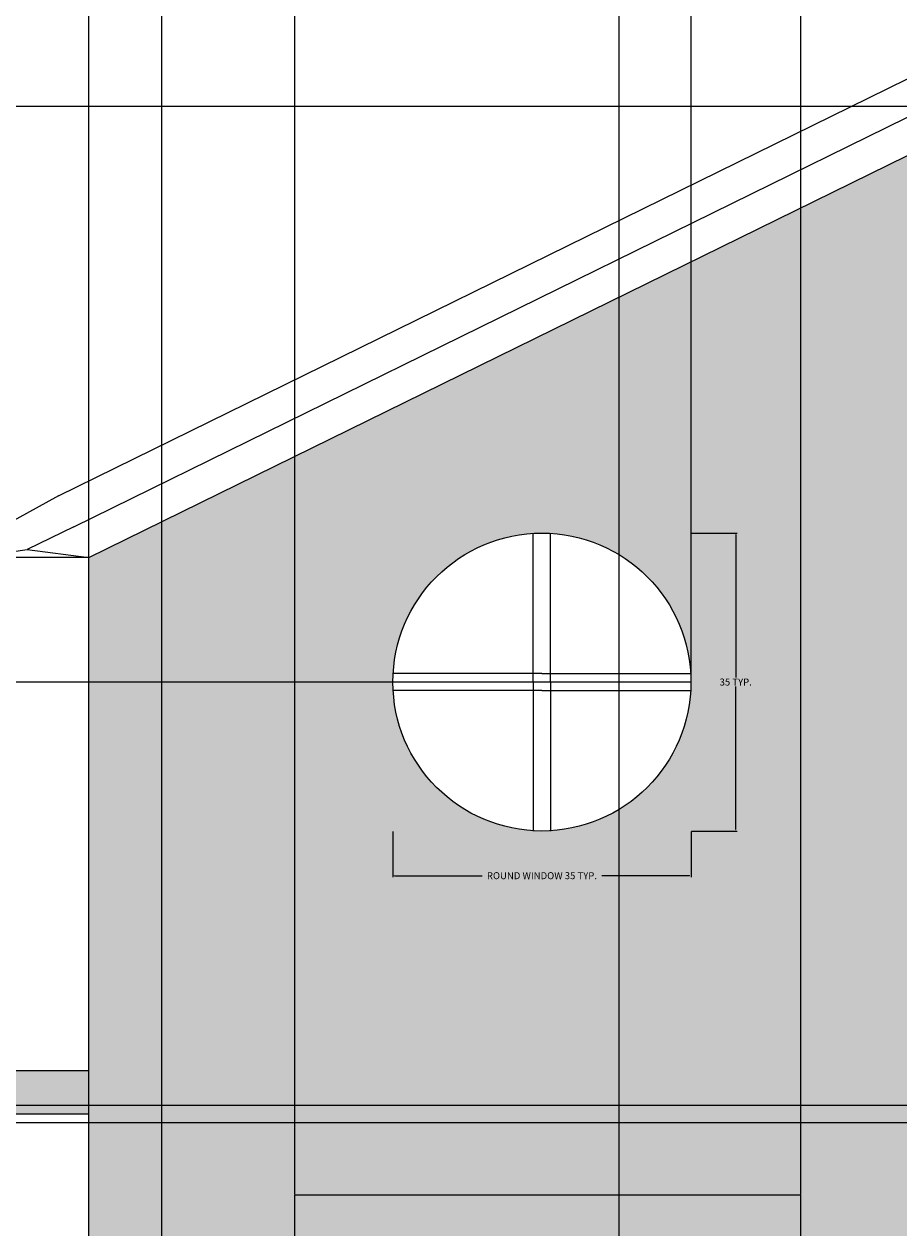
# Model space of a CAD drawing. Units: inches. Extents: x 36 to 594, y 79 to 831.
# Tile 21 of 30: x 87 to 189, y 590 to 730. Entities that reach past the tile are written whole.
import ezdxf

# ---------------------------------------------------------------- set-up
doc = ezdxf.new("R2010")
doc.units = ezdxf.units.IN
doc.header["$MEASUREMENT"] = 0
for name, color, linetype, lineweight in [('A-ANNO-DIMS', 2, 'Continuous', 18), ('A-ELEV', 7, 'Continuous', 25), ('A-ELEV-PATT', 8, 'Continuous', 13), ('A-GLAZ', 4, 'Continuous', 18)]:
    doc.layers.add(name, color=color, linetype=linetype, lineweight=lineweight)
doc.styles.get("Standard").update_dxf_attribs({"font": 'arial.ttf'})
doc.dimstyles.get("Standard").update_dxf_attribs({"dimtxt": 0.8125, "dimasz": 0.18, "dimexe": 0.18, "dimexo": 0.0625, "dimgap": 0.09, "dimtad": 0, "dimtih": 1, "dimtoh": 1, "dimdec": 4, "dimzin": 0, "dimdsep": 46, "dimlunit": 4, "dimtxsty": 'Standard', "dimcen": 0.09, "dimadec": 0, "dimazin": 0, "dimtfac": 1, "dimtdec": 4, "dimtofl": 0, "dimtmove": 0, "dimatfit": 3, "dimfxl": 1, "dimtolj": 1, "dimtzin": 0, "dimarcsym": 0})

# ---------------------------------------------------------------- blocks, each defined once
blk = doc.blocks.new('WIN-ROUND')
for p, q in [((146.46, 653.76), (146.46, 671.07)), ((148.46, 653.76), (148.46, 671.07)), ((147.46, 654.76), (130.16, 654.76)), ((147.46, 654.76), (164.77, 654.76)), ((146.46, 653.76), (146.46, 636.46)), ((148.46, 653.76), (148.46, 636.46)), ((147.46, 652.76), (130.16, 652.76)), ((147.46, 652.76), (164.77, 652.76))]:
    blk.add_line(p, q)
blk.add_circle((147.46, 653.76), 17.3)
blk = doc.blocks.new('*D5')
at = {"layer": 'A-ANNO-DIMS', "color": 0, "lineweight": -2, "transparency": 16777216}
for p, q in [((130.16, 636.4), (130.16, 631.09)), ((164.77, 636.4), (164.77, 631.09)), ((130.34, 631.27), (140.53, 631.27)), ((164.59, 631.27), (154.4, 631.27))]:
    blk.add_line(p, q, dxfattribs=at)
at = {"layer": 'A-ANNO-DIMS', "color": 0, "transparency": 16777216}
for points in [[(130.34, 631.3), (130.34, 631.24), (130.16, 631.27)], [(164.59, 631.3), (164.59, 631.24), (164.77, 631.27)]]:
    blk.add_solid(points, dxfattribs=at)
at = {"layer": 'Defpoints', "color": 0, "transparency": 16777216}
for p in [(130.16, 636.46), (164.77, 636.46), (164.77, 631.27)]:
    blk.add_point(p, dxfattribs=at)
at = {"layer": 'A-ANNO-DIMS', "color": 0, "transparency": 16777216, "insert": (147.46, 631.27), "char_height": 0.8125, "attachment_point": 5}
blk.add_mtext('\\A1;ROUND WINDOW 35 TYP.', dxfattribs=at)
blk = doc.blocks.new('*D6')
at = {"layer": 'A-ANNO-DIMS', "color": 0, "lineweight": -2, "transparency": 16777216}
for p, q in [((164.83, 671.07), (170.14, 671.07)), ((169.96, 670.89), (169.96, 654.27)), ((169.96, 636.64), (169.96, 653.26)), ((164.83, 636.46), (170.14, 636.46))]:
    blk.add_line(p, q, dxfattribs=at)
at = {"layer": 'A-ANNO-DIMS', "color": 0, "transparency": 16777216}
for points in [[(169.93, 670.89), (169.99, 670.89), (169.96, 671.07)], [(169.93, 636.64), (169.99, 636.64), (169.96, 636.46)]]:
    blk.add_solid(points, dxfattribs=at)
at = {"layer": 'Defpoints', "color": 0, "transparency": 16777216}
for p in [(164.77, 671.07), (169.96, 671.07), (164.77, 636.46)]:
    blk.add_point(p, dxfattribs=at)
at = {"layer": 'A-ANNO-DIMS', "color": 0, "transparency": 16777216, "insert": (169.96, 653.76), "char_height": 0.8125, "attachment_point": 5}
blk.add_mtext('\\A1;35 TYP.', dxfattribs=at)
blk = doc.blocks.new('*D12')
at = {"layer": 'A-ANNO-DIMS', "color": 0, "lineweight": -2, "transparency": 16777216}
for p, q in [((77.48, 667.8), (77.48, 830.73)), ((77.66, 830.55), (96.64, 830.55)), ((118.58, 830.55), (99.6, 830.55)), ((118.76, 594.27), (118.76, 830.73))]:
    blk.add_line(p, q, dxfattribs=at)
at = {"layer": 'A-ANNO-DIMS', "color": 0, "transparency": 16777216}
for points in [[(77.66, 830.58), (77.66, 830.52), (77.48, 830.55)], [(118.58, 830.58), (118.58, 830.52), (118.76, 830.55)]]:
    blk.add_solid(points, dxfattribs=at)
at = {"layer": 'Defpoints', "color": 0, "transparency": 16777216}
for p in [(118.76, 830.55), (77.48, 667.73), (118.76, 594.21)]:
    blk.add_point(p, dxfattribs=at)
at = {"layer": 'A-ANNO-DIMS', "color": 0, "transparency": 16777216, "insert": (98.12, 830.55), "char_height": 0.812, "attachment_point": 5}
blk.add_mtext('\\A1;41.28', dxfattribs=at)
blk = doc.blocks.new('*D13')
at = {"layer": 'A-ANNO-DIMS', "color": 0, "lineweight": -2, "transparency": 16777216}
for p, q in [((118.76, 594.27), (118.76, 830.73)), ((118.94, 830.55), (146.68, 830.55)), ((177.34, 830.55), (149.6, 830.55)), ((177.52, 594.27), (177.52, 830.73))]:
    blk.add_line(p, q, dxfattribs=at)
at = {"layer": 'A-ANNO-DIMS', "color": 0, "transparency": 16777216}
for points in [[(118.94, 830.58), (118.94, 830.52), (118.76, 830.55)], [(177.34, 830.58), (177.34, 830.52), (177.52, 830.55)]]:
    blk.add_solid(points, dxfattribs=at)
at = {"layer": 'Defpoints', "color": 0, "transparency": 16777216}
for p in [(177.52, 830.55), (118.76, 594.21), (177.52, 594.21)]:
    blk.add_point(p, dxfattribs=at)
at = {"layer": 'A-ANNO-DIMS', "color": 0, "transparency": 16777216, "insert": (148.14, 830.55), "char_height": 0.812, "attachment_point": 5}
blk.add_mtext('\\A1;58.77', dxfattribs=at)
blk = doc.blocks.new('*D14')
at = {"layer": 'A-ANNO-DIMS', "color": 0, "lineweight": -2, "transparency": 16777216}
for p, q in [((177.52, 594.27), (177.52, 830.73)), ((177.7, 830.55), (187.69, 830.55)), ((201.24, 830.55), (191.25, 830.55)), ((201.42, 720.66), (201.42, 830.73))]:
    blk.add_line(p, q, dxfattribs=at)
at = {"layer": 'A-ANNO-DIMS', "color": 0, "transparency": 16777216}
for points in [[(177.7, 830.58), (177.7, 830.52), (177.52, 830.55)], [(201.24, 830.58), (201.24, 830.52), (201.42, 830.55)]]:
    blk.add_solid(points, dxfattribs=at)
at = {"layer": 'Defpoints', "color": 0, "transparency": 16777216}
for p in [(201.42, 830.55), (201.42, 720.59), (177.52, 594.21)]:
    blk.add_point(p, dxfattribs=at)
at = {"layer": 'A-ANNO-DIMS', "color": 0, "transparency": 16777216, "insert": (189.47, 830.55), "char_height": 0.812, "attachment_point": 5}
blk.add_mtext('\\A1;23.894', dxfattribs=at)
blk = doc.blocks.new('*D21')
at = {"layer": 'A-ANNO-DIMS', "color": 0, "lineweight": -2, "transparency": 16777216}
for p, q in [((77.48, 667.8), (77.48, 830.73)), ((77.66, 830.55), (84.75, 830.55)), ((94.69, 830.55), (87.59, 830.55)), ((94.87, 668.27), (94.87, 830.73))]:
    blk.add_line(p, q, dxfattribs=at)
at = {"layer": 'A-ANNO-DIMS', "color": 0, "transparency": 16777216}
for points in [[(77.66, 830.58), (77.66, 830.52), (77.48, 830.55)], [(94.69, 830.58), (94.69, 830.52), (94.87, 830.55)]]:
    blk.add_solid(points, dxfattribs=at)
at = {"layer": 'Defpoints', "color": 0, "transparency": 16777216}
for p in [(94.87, 830.55), (77.48, 667.73), (94.87, 668.21)]:
    blk.add_point(p, dxfattribs=at)
at = {"layer": 'A-ANNO-DIMS', "color": 0, "transparency": 16777216, "insert": (86.17, 830.55), "char_height": 0.812, "attachment_point": 5}
blk.add_mtext('\\A1;17.39', dxfattribs=at)
blk = doc.blocks.new('*D27')
at = {"layer": 'A-ANNO-DIMS', "color": 0, "lineweight": -2, "transparency": 16777216}
for p, q in [((94.87, 668.27), (94.87, 830.73)), ((95.05, 830.55), (128.67, 830.55)), ((164.59, 830.55), (130.96, 830.55)), ((164.77, 653.83), (164.77, 830.73))]:
    blk.add_line(p, q, dxfattribs=at)
at = {"layer": 'A-ANNO-DIMS', "color": 0, "transparency": 16777216}
for points in [[(95.05, 830.58), (95.05, 830.52), (94.87, 830.55)], [(164.59, 830.58), (164.59, 830.52), (164.77, 830.55)]]:
    blk.add_solid(points, dxfattribs=at)
at = {"layer": 'Defpoints', "color": 0, "transparency": 16777216}
for p in [(164.77, 830.55), (94.87, 668.21), (164.77, 653.76)]:
    blk.add_point(p, dxfattribs=at)
at = {"layer": 'A-ANNO-DIMS', "color": 0, "transparency": 16777216, "insert": (129.82, 830.55), "char_height": 0.812, "attachment_point": 5}
blk.add_mtext('\\A1;69.9', dxfattribs=at)
blk = doc.blocks.new('*D28')
at = {"layer": 'A-ANNO-DIMS', "color": 0, "lineweight": -2, "transparency": 16777216}
for p, q in [((269.3, 796.05), (37.49, 796.05)), ((37.67, 795.87), (37.67, 455.63)), ((37.67, 114.39), (37.67, 454.62)), ((94.8, 114.21), (37.49, 114.21))]:
    blk.add_line(p, q, dxfattribs=at)
at = {"layer": 'A-ANNO-DIMS', "color": 0, "transparency": 16777216}
for points in [[(37.64, 795.87), (37.7, 795.87), (37.67, 796.05)], [(37.64, 114.39), (37.7, 114.39), (37.67, 114.21)]]:
    blk.add_solid(points, dxfattribs=at)
at = {"layer": 'Defpoints', "color": 0, "transparency": 16777216}
for p in [(37.67, 796.05), (269.36, 796.05), (94.87, 114.21)]:
    blk.add_point(p, dxfattribs=at)
at = {"layer": 'A-ANNO-DIMS', "color": 0, "transparency": 16777216, "insert": (37.67, 455.13), "char_height": 0.812, "attachment_point": 5}
blk.add_mtext('\\A1;681.8', dxfattribs=at)
blk = doc.blocks.new('*D46')
at = {"layer": 'A-ANNO-DIMS', "color": 0, "lineweight": -2, "transparency": 16777216}
for p, q in [((164.7, 653.76), (37.49, 653.76)), ((37.67, 653.58), (37.67, 631.69)), ((37.67, 608.79), (37.67, 630.68)), ((72.11, 608.61), (37.49, 608.61))]:
    blk.add_line(p, q, dxfattribs=at)
at = {"layer": 'A-ANNO-DIMS', "color": 0, "transparency": 16777216}
for points in [[(37.64, 653.58), (37.7, 653.58), (37.67, 653.76)], [(37.64, 608.79), (37.7, 608.79), (37.67, 608.61)]]:
    blk.add_solid(points, dxfattribs=at)
at = {"layer": 'Defpoints', "color": 0, "transparency": 16777216}
for p in [(37.67, 653.76), (164.77, 653.76), (72.17, 608.61)]:
    blk.add_point(p, dxfattribs=at)
at = {"layer": 'A-ANNO-DIMS', "color": 0, "transparency": 16777216, "insert": (37.67, 631.19), "char_height": 0.812, "attachment_point": 5}
blk.add_mtext('\\A1;45.16', dxfattribs=at)
blk = doc.blocks.new('*D47')
at = {"layer": 'A-ANNO-DIMS', "color": 0, "lineweight": -2, "transparency": 16777216}
for p, q in [((94.8, 668.21), (37.49, 668.21)), ((37.67, 668.03), (37.67, 661.49)), ((37.67, 653.94), (37.67, 660.48)), ((164.7, 653.76), (37.49, 653.76))]:
    blk.add_line(p, q, dxfattribs=at)
at = {"layer": 'A-ANNO-DIMS', "color": 0, "transparency": 16777216}
for points in [[(37.64, 668.03), (37.7, 668.03), (37.67, 668.21)], [(37.64, 653.94), (37.7, 653.94), (37.67, 653.76)]]:
    blk.add_solid(points, dxfattribs=at)
at = {"layer": 'Defpoints', "color": 0, "transparency": 16777216}
for p in [(37.67, 668.21), (94.87, 668.21), (164.77, 653.76)]:
    blk.add_point(p, dxfattribs=at)
at = {"layer": 'A-ANNO-DIMS', "color": 0, "transparency": 16777216, "insert": (37.67, 660.99), "char_height": 0.812, "attachment_point": 5}
blk.add_mtext('\\A1;14.448', dxfattribs=at)
blk = doc.blocks.new('*D48')
at = {"layer": 'A-ANNO-DIMS', "color": 0, "lineweight": -2, "transparency": 16777216}
for p, q in [((201.36, 720.59), (37.49, 720.59)), ((37.67, 720.41), (37.67, 694.91)), ((37.67, 668.39), (37.67, 693.9)), ((94.8, 668.21), (37.49, 668.21))]:
    blk.add_line(p, q, dxfattribs=at)
at = {"layer": 'A-ANNO-DIMS', "color": 0, "transparency": 16777216}
for points in [[(37.64, 720.41), (37.7, 720.41), (37.67, 720.59)], [(37.64, 668.39), (37.7, 668.39), (37.67, 668.21)]]:
    blk.add_solid(points, dxfattribs=at)
at = {"layer": 'Defpoints', "color": 0, "transparency": 16777216}
for p in [(37.67, 720.59), (201.42, 720.59), (94.87, 668.21)]:
    blk.add_point(p, dxfattribs=at)
at = {"layer": 'A-ANNO-DIMS', "color": 0, "transparency": 16777216, "insert": (37.67, 694.4), "char_height": 0.812, "attachment_point": 5}
blk.add_mtext('\\A1;52.38', dxfattribs=at)
blk = doc.blocks.new('*D49')
at = {"layer": 'A-ANNO-DIMS', "color": 0, "lineweight": -2, "transparency": 16777216}
for p, q in [((209.97, 733.74), (37.49, 733.74)), ((37.67, 733.56), (37.67, 727.67)), ((37.67, 720.77), (37.67, 726.66)), ((201.36, 720.59), (37.49, 720.59))]:
    blk.add_line(p, q, dxfattribs=at)
at = {"layer": 'A-ANNO-DIMS', "color": 0, "transparency": 16777216}
for points in [[(37.64, 733.56), (37.7, 733.56), (37.67, 733.74)], [(37.64, 720.77), (37.7, 720.77), (37.67, 720.59)]]:
    blk.add_solid(points, dxfattribs=at)
at = {"layer": 'Defpoints', "color": 0, "transparency": 16777216}
for p in [(37.67, 733.74), (210.03, 733.74), (201.42, 720.59)]:
    blk.add_point(p, dxfattribs=at)
at = {"layer": 'A-ANNO-DIMS', "color": 0, "transparency": 16777216, "insert": (37.67, 727.17), "char_height": 0.812, "attachment_point": 5}
blk.add_mtext('\\A1;13.147', dxfattribs=at)
blk = doc.blocks.new('*D60')
at = {"layer": 'A-ANNO-DIMS', "color": 0, "lineweight": -2, "transparency": 16777216}
for p, q in [((103.34, 286.24), (103.34, 830.73)), ((103.52, 830.55), (128.41, 830.55)), ((156.23, 830.55), (131.33, 830.55)), ((156.41, 264.68), (156.41, 830.73))]:
    blk.add_line(p, q, dxfattribs=at)
at = {"layer": 'A-ANNO-DIMS', "color": 0, "transparency": 16777216}
for points in [[(103.52, 830.58), (103.52, 830.52), (103.34, 830.55)], [(156.23, 830.58), (156.23, 830.52), (156.41, 830.55)]]:
    blk.add_solid(points, dxfattribs=at)
at = {"layer": 'Defpoints', "color": 0, "transparency": 16777216}
for p in [(156.41, 830.55), (103.34, 286.18), (156.41, 264.62)]:
    blk.add_point(p, dxfattribs=at)
at = {"layer": 'A-ANNO-DIMS', "color": 0, "transparency": 16777216, "insert": (129.87, 830.55), "char_height": 0.812, "attachment_point": 5}
blk.add_mtext('\\A1;53.07', dxfattribs=at)
blk = doc.blocks.new('*D61')
at = {"layer": 'A-ANNO-DIMS', "color": 0, "lineweight": -2, "transparency": 16777216}
for p, q in [((156.41, 264.68), (156.41, 830.73)), ((156.59, 830.55), (185.26, 830.55)), ((216.85, 830.55), (188.18, 830.55)), ((217.03, 286.24), (217.03, 830.73))]:
    blk.add_line(p, q, dxfattribs=at)
at = {"layer": 'A-ANNO-DIMS', "color": 0, "transparency": 16777216}
for points in [[(156.59, 830.58), (156.59, 830.52), (156.41, 830.55)], [(216.85, 830.58), (216.85, 830.52), (217.03, 830.55)]]:
    blk.add_solid(points, dxfattribs=at)
at = {"layer": 'Defpoints', "color": 0, "transparency": 16777216}
for p in [(217.03, 830.55), (217.03, 286.18), (156.41, 264.62)]:
    blk.add_point(p, dxfattribs=at)
at = {"layer": 'A-ANNO-DIMS', "color": 0, "transparency": 16777216, "insert": (186.72, 830.55), "char_height": 0.812, "attachment_point": 5}
blk.add_mtext('\\A1;60.62', dxfattribs=at)
blk = doc.blocks.new('*D122')
at = {"layer": 'A-ANNO-DIMS', "color": 0, "lineweight": -2, "transparency": 16777216}
for p, q in [((201.36, 604.57), (37.49, 604.57)), ((37.67, 604.39), (37.67, 604.06)), ((37.67, 602.75), (37.67, 603.07)), ((201.36, 602.57), (37.49, 602.57))]:
    blk.add_line(p, q, dxfattribs=at)
at = {"layer": 'A-ANNO-DIMS', "color": 0, "transparency": 16777216}
for points in [[(37.64, 604.39), (37.7, 604.39), (37.67, 604.57)], [(37.64, 602.75), (37.7, 602.75), (37.67, 602.57)]]:
    blk.add_solid(points, dxfattribs=at)
at = {"layer": 'Defpoints', "color": 0, "transparency": 16777216}
for p in [(37.67, 604.57), (201.42, 604.57), (201.42, 602.57)]:
    blk.add_point(p, dxfattribs=at)
at = {"layer": 'A-ANNO-DIMS', "color": 0, "transparency": 16777216, "insert": (37.67, 603.57), "char_height": 0.812, "attachment_point": 5}
blk.add_mtext('\\A1;2', dxfattribs=at)

msp = doc.modelspace()

# ---------------------------------------------------------------- hatches: boundary and pattern name
at = {"layer": 'A-ELEV-PATT'}
h = msp.add_hatch(color=256, dxfattribs=at)
h.dxf.hatch_style = 1
h.paths.add_polyline_path([(398.0873, 796.0465), (269.3592, 796.0465), (269.3592, 770.1455), (397.8159, 770.1455)])
h.paths.add_polyline_path([(397.7518, 764.0341), (269.3592, 764.0341), (269.3592, 630.0394), (341.8367, 630.0394), (341.8367, 720.595), (335.0881, 728.3699), (329.982, 735.3373), (345.3661, 727.7743), (397.1052, 702.3389)])
h.paths.add_polyline_path([(341.8367, 594.2124), (201.4189, 594.2124), (201.4189, 475.4136), (232.8216, 475.4136), (232.8216, 524.6037), (341.8367, 524.6037)])
h.paths.add_polyline_path([(177.525, 594.2124), (118.7598, 594.2124), (118.7598, 450.2124), (177.525, 450.2124)])
h.paths.add_polyline_path([(424.4958, 594.2124), (365.7306, 594.2124), (365.7306, 450.2124), (424.4958, 450.2124)])
h.paths.add_polyline_path([(241.3553, 404.2737), (355.8569, 404.2737), (355.8569, 355.0836), (424.5492, 355.0836), (424.5492, 425.7333), (118.7598, 426.2844), (118.7598, 355.0836), (241.3553, 355.0836)])
h.paths.add_polyline_path([(448.3898, 306.2124), (217.0273, 306.2124), (217.0273, 142.2124), (254.0293, 142.2124), (254.0293, 150.9347), (254.0293, 286.1802), (401.5491, 286.1802), (401.5491, 150.9347), (401.5491, 142.2124), (448.3898, 142.2124)])
h.paths.add_polyline_path([(448.3898, 142.2124), (401.5491, 142.2124), (217.0273, 142.2124), (217.0273, 114.2124), (448.3898, 114.2124)])
h.paths.add_polyline_path([(217.0273, 306.2124), (174.7353, 306.2124), (94.8658, 306.2124), (94.8658, 162.2124), (103.3368, 162.2124), (103.3368, 264.6224), (103.3368, 286.1802), (217.0273, 286.1802)])
h = msp.add_hatch(color=256, dxfattribs=at)
h.dxf.hatch_style = 1
h.paths.add_polyline_path([(94.8658, 608.6081), (72.1733, 608.6081), (72.1733, 603.598), (94.8658, 603.598)])
h.paths.add_polyline_path([(94.8658, 427.5982), (72.1733, 427.5982), (72.1733, 422.5882), (94.8658, 422.5882)])
h.paths.add_polyline_path([(94.8658, 299.486), (72.1733, 299.486), (72.1733, 294.4759), (94.8658, 294.4759)])
h.paths.add_polyline_path([(269.3592, 770.1455), (260.5727, 770.1455), (260.5727, 764.0341), (269.3592, 764.0341)])
h.paths.add_polyline_path([(410.2381, 770.1455), (269.3592, 770.1455), (269.3592, 764.0341), (410.2381, 764.0341)])
h = msp.add_hatch(color=256, dxfattribs=at)
h.dxf.hatch_style = 1
h.paths.add_polyline_path([(448.3898, 668.2124), (341.8367, 720.595), (341.8367, 594.2124), (341.8367, 450.2124), (365.7306, 450.2124), (365.7306, 594.2124), (424.4958, 594.2124), (424.4958, 450.2124), (448.3898, 450.2124), (448.3898, 594.2124)])
h.paths.add_polyline_path([(378.5958, 653.8563, -1), (413.2033, 653.8563, -1)], flags=16)
h.paths.add_polyline_path([(394.8995, 653.8563), (394.8995, 654.8563), (395.8995, 654.8563), (396.8995, 654.8563), (396.8995, 653.8563), (396.8995, 652.8563), (395.8995, 652.8563), (394.8995, 652.8563)], flags=0)
h.paths.add_polyline_path([(201.4189, 708.8485), (201.4189, 720.595), (94.8658, 668.2124), (94.8658, 644.2124), (94.8658, 596.2124), (94.8658, 594.2124), (94.8658, 450.2124), (118.7598, 450.2124), (118.7598, 594.2124), (177.525, 594.2124), (177.525, 450.2124), (201.4189, 450.2124), (201.4189, 594.2124)])
h.paths.add_polyline_path([(130.1589, 653.7648, -1), (164.7665, 653.7648, -1)], flags=16)
h.paths.add_polyline_path([(148.4627, 652.7648), (147.4627, 652.7648), (146.4627, 652.7648), (146.4627, 653.7648), (146.4627, 654.7648), (147.4627, 654.7648), (148.4627, 654.7648), (148.4627, 653.7648)], flags=0)

# ---------------------------------------------------------------- linework, layer by layer
at = {"layer": 'A-ELEV'}
for p, q in [((91.3364, 675.3917), (197.8895, 727.7743)), ((93.1011, 671.802), (199.6542, 724.1846)), ((94.8658, 668.2124), (201.4189, 720.595)), ((91.3364, 675.3917), (77.477, 667.7335)), ((93.1011, 671.802), (87.7109, 669.1522)), ((77.477, 667.7335), (87.7109, 669.1522)), ((87.7109, 669.1522), (94.8658, 668.2124)), ((94.8658, 644.2124), (94.8658, 668.2124)), ((94.8658, 596.2124), (94.8658, 644.2124)), ((94.8658, 594.2124), (94.8658, 598.2124)), ((94.8658, 450.2124), (94.8658, 594.2124))]:
    msp.add_line(p, q, dxfattribs=at)
msp.add_lwpolyline([(94.8658, 608.6081), (72.1733, 608.6081), (72.1733, 603.598), (94.8658, 603.598)], close=True, dxfattribs=at)
at = {"layer": 'A-GLAZ'}
for p, q in [((118.7598, 450.2124), (118.7598, 594.2124)), ((118.7598, 594.2124), (177.525, 594.2124)), ((177.525, 450.2124), (177.525, 594.2124))]:
    msp.add_line(p, q, dxfattribs=at)

# ---------------------------------------------------------------- block references
msp.add_blockref('WIN-ROUND', (0, 0), dxfattribs=at)

# ---------------------------------------------------------------- dimensions: what is measured, and where the dimension line sits
at = {"layer": 'A-ANNO-DIMS'}
for base, p1, p2, override, picture, middle in [((118.7598, 830.5465), (77.477, 667.7335), (118.7598, 594.2124), {"dimdec": 2, "dimlfac": 1, "dimrnd": 0, "dimzin": 0, "dimdsep": 46, "dimlunit": 2}, '*D12', (98.1184, 830.5465)), ((94.8658, 830.5465), (77.477, 667.7335), (94.8658, 668.2124), {"dimdec": 2, "dimlfac": 1, "dimrnd": 0, "dimzin": 0, "dimdsep": 46, "dimlunit": 2}, '*D21', (86.1714, 830.5465)), ((164.7665, 830.5465), (94.8658, 668.2124), (164.7665, 653.7648), {"dimdec": 1, "dimlfac": 1, "dimrnd": 0, "dimzin": 0, "dimdsep": 46, "dimlunit": 2}, '*D27', (129.8161, 830.5465)), ((156.4069, 830.5465), (103.3368, 286.1802), (156.4069, 264.6224), {"dimdec": 2, "dimlfac": 1, "dimrnd": 0, "dimzin": 0, "dimdsep": 46, "dimlunit": 2}, '*D60', (129.8718, 830.5465)), ((177.525, 830.5465), (118.7598, 594.2124), (177.525, 594.2124), {"dimdec": 2, "dimlfac": 1, "dimrnd": 0, "dimzin": 0, "dimdsep": 46, "dimlunit": 2}, '*D13', (148.1424, 830.5465)), ((217.0273, 830.5465), (156.4069, 264.6224), (217.0273, 286.1802), {"dimdec": 2, "dimlfac": 1, "dimrnd": 0, "dimzin": 0, "dimdsep": 46, "dimlunit": 2}, '*D61', (186.7171, 830.5465)), ((201.4189, 830.5465), (177.525, 594.2124), (201.4189, 720.595), {"dimdec": 3, "dimlfac": 1, "dimrnd": 0, "dimzin": 0, "dimdsep": 46, "dimlunit": 2}, '*D14', (189.4719, 830.5465))]:
    dim = msp.add_linear_dim(base=base, p1=p1, p2=p2, dimstyle='Standard', override=override, dxfattribs=at)
    dim.commit()
    dim.dimension.update_dxf_attribs({"geometry": picture, "text_midpoint": middle})
for base, p1, p2, override, picture, middle in [((37.6733, 796.0465), (94.8658, 114.2124), (269.3592, 796.0465), {"dimdec": 1, "dimlfac": 1, "dimrnd": 0, "dimzin": 0, "dimdsep": 46, "dimlunit": 2}, '*D28', (37.6733, 455.1294)), ((37.6733, 733.7417), (201.4189, 720.595), (210.028, 733.7417), {"dimdec": 3, "dimlfac": 1, "dimrnd": 0, "dimzin": 0, "dimdsep": 46, "dimlunit": 2}, '*D49', (37.6733, 727.1683)), ((37.6733, 720.595), (94.8658, 668.2124), (201.4189, 720.595), {"dimdec": 2, "dimlfac": 1, "dimrnd": 0, "dimzin": 0, "dimdsep": 46, "dimlunit": 2}, '*D48', (37.6733, 694.4037)), ((37.6733, 668.2124), (164.7665, 653.7648), (94.8658, 668.2124), {"dimdec": 3, "dimlfac": 1, "dimrnd": 0, "dimzin": 0, "dimdsep": 46, "dimlunit": 2}, '*D47', (37.6733, 660.9886)), ((37.6733, 653.7648), (72.1733, 608.6081), (164.7665, 653.7648), {"dimdec": 2, "dimlfac": 1, "dimrnd": 0, "dimzin": 0, "dimdsep": 46, "dimlunit": 2}, '*D46', (37.6733, 631.1865)), ((37.6733, 604.5667), (201.4189, 602.5667), (201.4189, 604.5667), {"dimdec": 0, "dimlfac": 1, "dimrnd": 0, "dimzin": 0, "dimdsep": 46, "dimlunit": 2}, '*D122', (37.6733, 603.5667))]:
    dim = msp.add_linear_dim(base=base, p1=p1, p2=p2, angle=90, dimstyle='Standard', override=override, dxfattribs=at)
    dim.commit()
    dim.dimension.update_dxf_attribs({"geometry": picture, "text_midpoint": middle})
dim = msp.add_linear_dim(base=(169.9576, 671.0686), p1=(164.7665, 636.4611), p2=(164.7665, 671.0686), angle=90, text='<> TYP.', dimstyle='Standard', override={"dimdec": 0, "dimlfac": 1, "dimrnd": 0, "dimzin": 0, "dimdsep": 46, "dimlunit": 2}, dxfattribs=at)
dim.commit()
dim.dimension.update_dxf_attribs({"geometry": '*D6', "text_midpoint": (169.9576, 653.7648)})
dim = msp.add_linear_dim(base=(164.7665, 631.2699), p1=(130.1589, 636.4611), p2=(164.7665, 636.4611), text='ROUND WINDOW <> TYP.', dimstyle='Standard', override={"dimdec": 0, "dimlfac": 1, "dimrnd": 0, "dimzin": 0, "dimdsep": 46, "dimlunit": 2}, dxfattribs=at)
dim.commit()
dim.dimension.update_dxf_attribs({"geometry": '*D5', "text_midpoint": (147.4627, 631.2699)})

doc.saveas('drawing.dxf')
